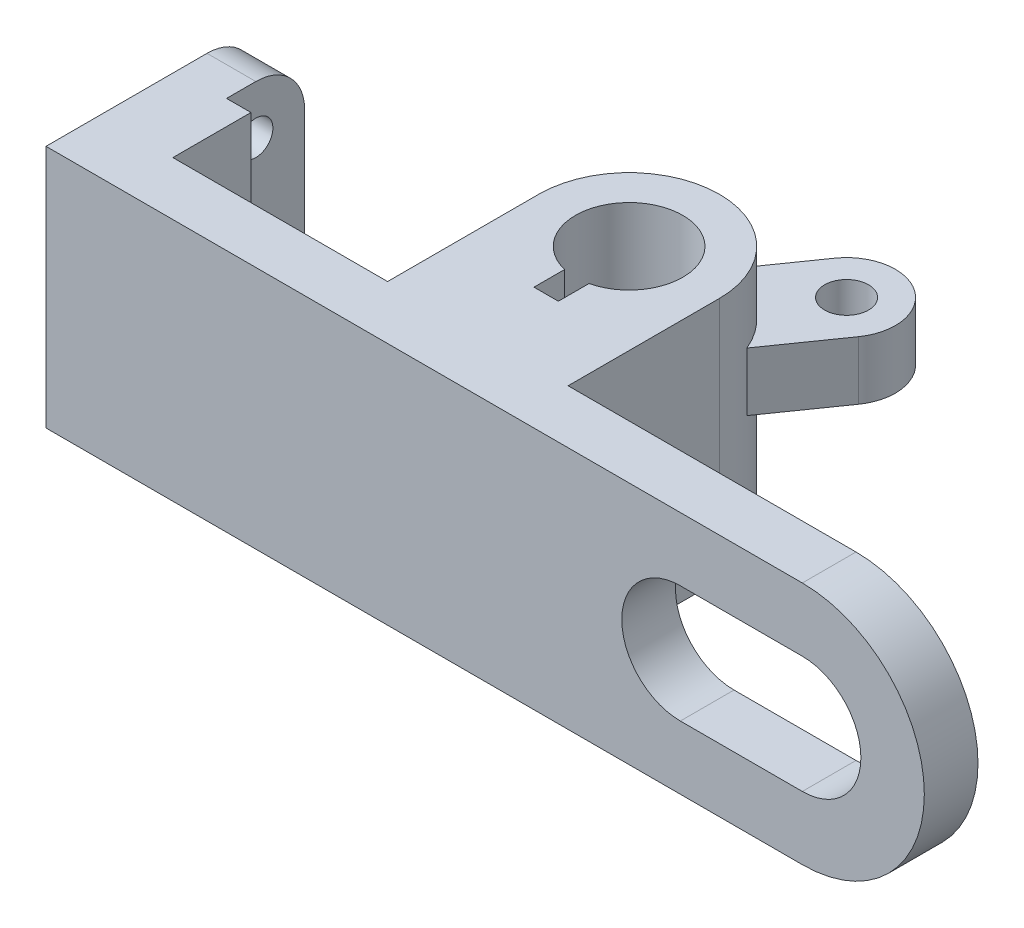
ISO-10303-21;
HEADER;
FILE_DESCRIPTION(('STEP AP214'),'2;1');
FILE_NAME('part.step','',(''),(''),'','','');
FILE_SCHEMA(('AUTOMOTIVE_DESIGN { 1 0 10303 214 1 1 1 1 }'));
ENDSEC;
DATA;
#1=APPLICATION_CONTEXT('core data for automotive mechanical design processes');
#2=APPLICATION_PROTOCOL_DEFINITION('international standard','automotive_design',2000,#1);
#3=PRODUCT_CONTEXT('',#1,'mechanical');
#4=PRODUCT('Part','Part','',(#3));
#5=PRODUCT_RELATED_PRODUCT_CATEGORY('part','',(#4));
#6=PRODUCT_DEFINITION_FORMATION('','',#4);
#7=PRODUCT_DEFINITION_CONTEXT('part definition',#1,'design');
#8=PRODUCT_DEFINITION('design','',#6,#7);
#9=PRODUCT_DEFINITION_SHAPE('','',#8);
#10=(LENGTH_UNIT() NAMED_UNIT(*) SI_UNIT(.MILLI.,.METRE.));
#11=(NAMED_UNIT(*) PLANE_ANGLE_UNIT() SI_UNIT($,.RADIAN.));
#12=(NAMED_UNIT(*) SI_UNIT($,.STERADIAN.) SOLID_ANGLE_UNIT());
#13=UNCERTAINTY_MEASURE_WITH_UNIT(LENGTH_MEASURE(1.E-05),#10,'distance_accuracy_value','');
#14=(GEOMETRIC_REPRESENTATION_CONTEXT(3) GLOBAL_UNCERTAINTY_ASSIGNED_CONTEXT((#13)) GLOBAL_UNIT_ASSIGNED_CONTEXT((#10,
#11,#12)) REPRESENTATION_CONTEXT('',''));
#15=CARTESIAN_POINT('',(0.,0.,0.));
#16=DIRECTION('',(0.,0.,1.));
#17=DIRECTION('',(1.,0.,0.));
#18=AXIS2_PLACEMENT_3D('',#15,#16,#17);
#19=CARTESIAN_POINT('',(0.,25.,-31.));
#20=DIRECTION('',(0.,-1.,0.));
#21=DIRECTION('',(0.,0.,-1.));
#22=AXIS2_PLACEMENT_3D('',#19,#20,#21);
#23=CYLINDRICAL_SURFACE('',#22,18.5);
#24=CARTESIAN_POINT('',(0.,-25.,-31.));
#25=DIRECTION('',(0.,1.,0.));
#26=DIRECTION('',(0.,0.,1.));
#27=AXIS2_PLACEMENT_3D('',#24,#25,#26);
#28=CIRCLE('',#27,18.5);
#29=CARTESIAN_POINT('',(18.5,-25.,-31.));
#30=VERTEX_POINT('',#29);
#31=CARTESIAN_POINT('',(-18.5,-25.,-31.));
#32=VERTEX_POINT('',#31);
#33=EDGE_CURVE('E290',#30,#32,#28,.T.);
#34=ORIENTED_EDGE('',*,*,#33,.T.);
#35=DIRECTION('',(0.,-1.,0.));
#36=VECTOR('',#35,1.);
#37=CARTESIAN_POINT('',(-18.5,25.,-31.));
#38=LINE('',#37,#36);
#39=CARTESIAN_POINT('',(-18.5,25.,-31.));
#40=VERTEX_POINT('',#39);
#41=EDGE_CURVE('E299',#40,#32,#38,.T.);
#42=ORIENTED_EDGE('',*,*,#41,.F.);
#43=CARTESIAN_POINT('',(0.,25.,-31.));
#44=DIRECTION('',(0.,1.,0.));
#45=DIRECTION('',(0.,0.,1.));
#46=AXIS2_PLACEMENT_3D('',#43,#44,#45);
#47=CIRCLE('',#46,18.5);
#48=CARTESIAN_POINT('',(18.5,25.,-31.));
#49=VERTEX_POINT('',#48);
#50=EDGE_CURVE('E270',#49,#40,#47,.T.);
#51=ORIENTED_EDGE('',*,*,#50,.F.);
#52=DIRECTION('',(0.,-1.,0.));
#53=VECTOR('',#52,1.);
#54=CARTESIAN_POINT('',(18.5,25.,-31.));
#55=LINE('',#54,#53);
#56=EDGE_CURVE('E301',#49,#30,#55,.T.);
#57=ORIENTED_EDGE('',*,*,#56,.T.);
#58=EDGE_LOOP('',(#34,#42,#51,#57));
#59=FACE_BOUND('',#58,.T.);
#60=DIRECTION('',(0.,-1.,0.));
#61=VECTOR('',#60,1.);
#62=CARTESIAN_POINT('',(17.1188834432209,12.,-38.0138313108756));
#63=LINE('',#62,#61);
#64=CARTESIAN_POINT('',(17.1188834432209,12.,-38.0138313108756));
#65=VERTEX_POINT('',#64);
#66=CARTESIAN_POINT('',(17.1188834432209,0.,-38.0138313108756));
#67=VERTEX_POINT('',#66);
#68=EDGE_CURVE('E59',#65,#67,#63,.T.);
#69=ORIENTED_EDGE('',*,*,#68,.F.);
#70=CARTESIAN_POINT('',(0.,12.,-31.));
#71=DIRECTION('',(0.,-1.,0.));
#72=DIRECTION('',(0.,0.,1.));
#73=AXIS2_PLACEMENT_3D('',#70,#71,#72);
#74=CIRCLE('',#73,18.5);
#75=CARTESIAN_POINT('',(0.735842557440977,12.,-49.4853600378965));
#76=VERTEX_POINT('',#75);
#77=EDGE_CURVE('E224',#76,#65,#74,.T.);
#78=ORIENTED_EDGE('',*,*,#77,.F.);
#79=DIRECTION('',(0.,-1.,0.));
#80=VECTOR('',#79,1.);
#81=CARTESIAN_POINT('',(0.735842557440977,12.,-49.4853600378965));
#82=LINE('',#81,#80);
#83=CARTESIAN_POINT('',(0.735842557440979,0.,-49.4853600378965));
#84=VERTEX_POINT('',#83);
#85=EDGE_CURVE('E240',#76,#84,#82,.T.);
#86=ORIENTED_EDGE('',*,*,#85,.T.);
#87=CARTESIAN_POINT('',(0.,0.,-31.));
#88=DIRECTION('',(0.,-1.,0.));
#89=DIRECTION('',(0.,0.,1.));
#90=AXIS2_PLACEMENT_3D('',#87,#88,#89);
#91=CIRCLE('',#90,18.5);
#92=EDGE_CURVE('E64',#84,#67,#91,.T.);
#93=ORIENTED_EDGE('',*,*,#92,.T.);
#94=EDGE_LOOP('',(#69,#78,#86,#93));
#95=FACE_BOUND('',#94,.T.);
#96=ADVANCED_FACE('F41',(#59,#95),#23,.T.);
#97=CARTESIAN_POINT('',(77.5,0.,0.));
#98=DIRECTION('',(0.,0.,1.));
#99=DIRECTION('',(1.,0.,0.));
#100=AXIS2_PLACEMENT_3D('',#97,#98,#99);
#101=PLANE('',#100);
#102=CARTESIAN_POINT('',(52.5,0.,0.));
#103=DIRECTION('',(0.,0.,1.));
#104=DIRECTION('',(1.,0.,0.));
#105=AXIS2_PLACEMENT_3D('',#102,#103,#104);
#106=CIRCLE('',#105,12.);
#107=CARTESIAN_POINT('',(52.5,12.,0.));
#108=VERTEX_POINT('',#107);
#109=CARTESIAN_POINT('',(52.5,-12.,0.));
#110=VERTEX_POINT('',#109);
#111=EDGE_CURVE('E347',#108,#110,#106,.T.);
#112=ORIENTED_EDGE('',*,*,#111,.T.);
#113=DIRECTION('',(1.,0.,0.));
#114=VECTOR('',#113,1.);
#115=CARTESIAN_POINT('',(52.5,-12.,0.));
#116=LINE('',#115,#114);
#117=CARTESIAN_POINT('',(77.5,-12.,0.));
#118=VERTEX_POINT('',#117);
#119=EDGE_CURVE('E359',#110,#118,#116,.T.);
#120=ORIENTED_EDGE('',*,*,#119,.T.);
#121=CARTESIAN_POINT('',(77.5,0.,0.));
#122=DIRECTION('',(0.,0.,1.));
#123=DIRECTION('',(1.,0.,0.));
#124=AXIS2_PLACEMENT_3D('',#121,#122,#123);
#125=CIRCLE('',#124,12.);
#126=CARTESIAN_POINT('',(77.5,12.,0.));
#127=VERTEX_POINT('',#126);
#128=EDGE_CURVE('E361',#118,#127,#125,.T.);
#129=ORIENTED_EDGE('',*,*,#128,.T.);
#130=DIRECTION('',(-1.,0.,0.));
#131=VECTOR('',#130,1.);
#132=CARTESIAN_POINT('',(52.5,12.,0.));
#133=LINE('',#132,#131);
#134=EDGE_CURVE('E348',#127,#108,#133,.T.);
#135=ORIENTED_EDGE('',*,*,#134,.T.);
#136=EDGE_LOOP('',(#112,#120,#129,#135));
#137=FACE_BOUND('',#136,.T.);
#138=DIRECTION('',(0.,-1.,0.));
#139=VECTOR('',#138,1.);
#140=CARTESIAN_POINT('',(18.5,25.,0.));
#141=LINE('',#140,#139);
#142=CARTESIAN_POINT('',(18.5,25.,0.));
#143=VERTEX_POINT('',#142);
#144=CARTESIAN_POINT('',(18.5,-25.,0.));
#145=VERTEX_POINT('',#144);
#146=EDGE_CURVE('E291',#143,#145,#141,.T.);
#147=ORIENTED_EDGE('',*,*,#146,.F.);
#148=DIRECTION('',(-1.,0.,0.));
#149=VECTOR('',#148,1.);
#150=CARTESIAN_POINT('',(-77.5,25.,0.));
#151=LINE('',#150,#149);
#152=CARTESIAN_POINT('',(77.5,25.0000000000001,0.));
#153=VERTEX_POINT('',#152);
#154=EDGE_CURVE('E385',#153,#143,#151,.T.);
#155=ORIENTED_EDGE('',*,*,#154,.F.);
#156=CARTESIAN_POINT('',(77.5,0.,0.));
#157=DIRECTION('',(0.,0.,1.));
#158=DIRECTION('',(1.,0.,0.));
#159=AXIS2_PLACEMENT_3D('',#156,#157,#158);
#160=CIRCLE('',#159,25.);
#161=CARTESIAN_POINT('',(77.5,-25.,0.));
#162=VERTEX_POINT('',#161);
#163=EDGE_CURVE('E395',#162,#153,#160,.T.);
#164=ORIENTED_EDGE('',*,*,#163,.F.);
#165=DIRECTION('',(1.,0.,0.));
#166=VECTOR('',#165,1.);
#167=CARTESIAN_POINT('',(-77.5,-25.,0.));
#168=LINE('',#167,#166);
#169=EDGE_CURVE('E380',#145,#162,#168,.T.);
#170=ORIENTED_EDGE('',*,*,#169,.F.);
#171=EDGE_LOOP('',(#147,#155,#164,#170));
#172=FACE_BOUND('',#171,.T.);
#173=ADVANCED_FACE('F480',(#137,#172),#101,.F.);
#174=CARTESIAN_POINT('',(-18.5,25.,0.));
#175=VERTEX_POINT('',#174);
#176=CARTESIAN_POINT('',(-62.5,25.,0.));
#177=VERTEX_POINT('',#176);
#178=EDGE_CURVE('E391',#175,#177,#151,.T.);
#179=ORIENTED_EDGE('',*,*,#178,.F.);
#180=DIRECTION('',(0.,-1.,0.));
#181=VECTOR('',#180,1.);
#182=CARTESIAN_POINT('',(-18.5,25.,0.));
#183=LINE('',#182,#181);
#184=CARTESIAN_POINT('',(-18.5,-25.,0.));
#185=VERTEX_POINT('',#184);
#186=EDGE_CURVE('E294',#175,#185,#183,.T.);
#187=ORIENTED_EDGE('',*,*,#186,.T.);
#188=CARTESIAN_POINT('',(-62.5,-25.,0.));
#189=VERTEX_POINT('',#188);
#190=EDGE_CURVE('E386',#189,#185,#168,.T.);
#191=ORIENTED_EDGE('',*,*,#190,.F.);
#192=DIRECTION('',(0.,-1.,0.));
#193=VECTOR('',#192,1.);
#194=CARTESIAN_POINT('',(-62.5,25.,0.));
#195=LINE('',#194,#193);
#196=EDGE_CURVE('E344',#177,#189,#195,.T.);
#197=ORIENTED_EDGE('',*,*,#196,.F.);
#198=EDGE_LOOP('',(#179,#187,#191,#197));
#199=FACE_BOUND('',#198,.T.);
#200=ADVANCED_FACE('F489',(#199),#101,.F.);
#201=CARTESIAN_POINT('',(77.5,0.,11.));
#202=DIRECTION('',(0.,0.,1.));
#203=DIRECTION('',(1.,0.,0.));
#204=AXIS2_PLACEMENT_3D('',#201,#202,#203);
#205=PLANE('',#204);
#206=DIRECTION('',(0.,-1.,0.));
#207=VECTOR('',#206,1.);
#208=CARTESIAN_POINT('',(-77.5,25.,11.));
#209=LINE('',#208,#207);
#210=CARTESIAN_POINT('',(-77.5,25.,11.));
#211=VERTEX_POINT('',#210);
#212=CARTESIAN_POINT('',(-77.5,-25.,11.));
#213=VERTEX_POINT('',#212);
#214=EDGE_CURVE('E377',#211,#213,#209,.T.);
#215=ORIENTED_EDGE('',*,*,#214,.T.);
#216=DIRECTION('',(1.,0.,0.));
#217=VECTOR('',#216,1.);
#218=CARTESIAN_POINT('',(-77.5,-25.,11.));
#219=LINE('',#218,#217);
#220=CARTESIAN_POINT('',(77.5,-25.,11.));
#221=VERTEX_POINT('',#220);
#222=EDGE_CURVE('E382',#213,#221,#219,.T.);
#223=ORIENTED_EDGE('',*,*,#222,.T.);
#224=CARTESIAN_POINT('',(77.5,0.,11.));
#225=DIRECTION('',(0.,0.,1.));
#226=DIRECTION('',(1.,0.,0.));
#227=AXIS2_PLACEMENT_3D('',#224,#225,#226);
#228=CIRCLE('',#227,25.);
#229=CARTESIAN_POINT('',(77.5,25.0000000000001,11.));
#230=VERTEX_POINT('',#229);
#231=EDGE_CURVE('E381',#221,#230,#228,.T.);
#232=ORIENTED_EDGE('',*,*,#231,.T.);
#233=DIRECTION('',(-1.,0.,0.));
#234=VECTOR('',#233,1.);
#235=CARTESIAN_POINT('',(-77.5,25.,11.));
#236=LINE('',#235,#234);
#237=EDGE_CURVE('E387',#230,#211,#236,.T.);
#238=ORIENTED_EDGE('',*,*,#237,.T.);
#239=EDGE_LOOP('',(#215,#223,#232,#238));
#240=FACE_BOUND('',#239,.T.);
#241=DIRECTION('',(1.,0.,0.));
#242=VECTOR('',#241,1.);
#243=CARTESIAN_POINT('',(52.5,-12.,11.));
#244=LINE('',#243,#242);
#245=CARTESIAN_POINT('',(52.5,-12.,11.));
#246=VERTEX_POINT('',#245);
#247=CARTESIAN_POINT('',(77.5,-12.,11.));
#248=VERTEX_POINT('',#247);
#249=EDGE_CURVE('E346',#246,#248,#244,.T.);
#250=ORIENTED_EDGE('',*,*,#249,.F.);
#251=CARTESIAN_POINT('',(52.5,0.,11.));
#252=DIRECTION('',(0.,0.,1.));
#253=DIRECTION('',(1.,0.,0.));
#254=AXIS2_PLACEMENT_3D('',#251,#252,#253);
#255=CIRCLE('',#254,12.);
#256=CARTESIAN_POINT('',(52.5,12.,11.));
#257=VERTEX_POINT('',#256);
#258=EDGE_CURVE('E350',#257,#246,#255,.T.);
#259=ORIENTED_EDGE('',*,*,#258,.F.);
#260=DIRECTION('',(-1.,0.,0.));
#261=VECTOR('',#260,1.);
#262=CARTESIAN_POINT('',(52.5,12.,11.));
#263=LINE('',#262,#261);
#264=CARTESIAN_POINT('',(77.5,12.,11.));
#265=VERTEX_POINT('',#264);
#266=EDGE_CURVE('E352',#265,#257,#263,.T.);
#267=ORIENTED_EDGE('',*,*,#266,.F.);
#268=CARTESIAN_POINT('',(77.5,0.,11.));
#269=DIRECTION('',(0.,0.,1.));
#270=DIRECTION('',(1.,0.,0.));
#271=AXIS2_PLACEMENT_3D('',#268,#269,#270);
#272=CIRCLE('',#271,12.);
#273=EDGE_CURVE('E351',#248,#265,#272,.T.);
#274=ORIENTED_EDGE('',*,*,#273,.F.);
#275=EDGE_LOOP('',(#250,#259,#267,#274));
#276=FACE_BOUND('',#275,.T.);
#277=ADVANCED_FACE('F437',(#240,#276),#205,.T.);
#278=CARTESIAN_POINT('',(-77.5,25.,11.));
#279=DIRECTION('',(1.,0.,0.));
#280=DIRECTION('',(0.,0.,-1.));
#281=AXIS2_PLACEMENT_3D('',#278,#279,#280);
#282=PLANE('',#281);
#283=CARTESIAN_POINT('',(-77.5,15.,-22.));
#284=DIRECTION('',(1.,0.,0.));
#285=DIRECTION('',(0.,0.,-1.));
#286=AXIS2_PLACEMENT_3D('',#283,#284,#285);
#287=CIRCLE('',#286,3.5);
#288=CARTESIAN_POINT('',(-77.5,15.,-25.5));
#289=VERTEX_POINT('',#288);
#290=EDGE_CURVE('E313',#289,#289,#287,.T.);
#291=ORIENTED_EDGE('',*,*,#290,.T.);
#292=EDGE_LOOP('',(#291));
#293=FACE_BOUND('',#292,.T.);
#294=CARTESIAN_POINT('',(-77.5,-15.,-22.));
#295=DIRECTION('',(1.,0.,0.));
#296=DIRECTION('',(0.,0.,-1.));
#297=AXIS2_PLACEMENT_3D('',#294,#295,#296);
#298=CIRCLE('',#297,3.5);
#299=CARTESIAN_POINT('',(-77.5,-15.,-25.5));
#300=VERTEX_POINT('',#299);
#301=EDGE_CURVE('E311',#300,#300,#298,.T.);
#302=ORIENTED_EDGE('',*,*,#301,.T.);
#303=EDGE_LOOP('',(#302));
#304=FACE_BOUND('',#303,.T.);
#305=DIRECTION('',(0.,0.,-1.));
#306=VECTOR('',#305,1.);
#307=CARTESIAN_POINT('',(-77.5,25.,11.));
#308=LINE('',#307,#306);
#309=CARTESIAN_POINT('',(-77.5,25.,-22.));
#310=VERTEX_POINT('',#309);
#311=EDGE_CURVE('E389',#211,#310,#308,.T.);
#312=ORIENTED_EDGE('',*,*,#311,.T.);
#313=CARTESIAN_POINT('',(-77.5,15.,-22.));
#314=DIRECTION('',(1.,0.,0.));
#315=DIRECTION('',(0.,0.,-1.));
#316=AXIS2_PLACEMENT_3D('',#313,#314,#315);
#317=CIRCLE('',#316,10.);
#318=CARTESIAN_POINT('',(-77.5,15.,-32.));
#319=VERTEX_POINT('',#318);
#320=EDGE_CURVE('E414',#310,#319,#317,.F.);
#321=ORIENTED_EDGE('',*,*,#320,.T.);
#322=DIRECTION('',(0.,-1.,0.));
#323=VECTOR('',#322,1.);
#324=CARTESIAN_POINT('',(-77.5,25.,-32.));
#325=LINE('',#324,#323);
#326=CARTESIAN_POINT('',(-77.5,-15.,-32.));
#327=VERTEX_POINT('',#326);
#328=EDGE_CURVE('E327',#319,#327,#325,.T.);
#329=ORIENTED_EDGE('',*,*,#328,.T.);
#330=CARTESIAN_POINT('',(-77.5,-15.,-22.));
#331=DIRECTION('',(1.,0.,0.));
#332=DIRECTION('',(0.,0.,-1.));
#333=AXIS2_PLACEMENT_3D('',#330,#331,#332);
#334=CIRCLE('',#333,10.);
#335=CARTESIAN_POINT('',(-77.5,-25.,-22.));
#336=VERTEX_POINT('',#335);
#337=EDGE_CURVE('E412',#327,#336,#334,.F.);
#338=ORIENTED_EDGE('',*,*,#337,.T.);
#339=DIRECTION('',(0.,0.,-1.));
#340=VECTOR('',#339,1.);
#341=CARTESIAN_POINT('',(-77.5,-25.,11.));
#342=LINE('',#341,#340);
#343=EDGE_CURVE('E403',#213,#336,#342,.T.);
#344=ORIENTED_EDGE('',*,*,#343,.F.);
#345=ORIENTED_EDGE('',*,*,#214,.F.);
#346=EDGE_LOOP('',(#312,#321,#329,#338,#344,#345));
#347=FACE_BOUND('',#346,.T.);
#348=ADVANCED_FACE('F434',(#293,#304,#347),#282,.F.);
#349=CARTESIAN_POINT('',(-77.5,-25.,11.));
#350=DIRECTION('',(0.,1.,0.));
#351=DIRECTION('',(-1.,0.,0.));
#352=AXIS2_PLACEMENT_3D('',#349,#350,#351);
#353=PLANE('',#352);
#354=ORIENTED_EDGE('',*,*,#343,.T.);
#355=DIRECTION('',(-1.,0.,0.));
#356=VECTOR('',#355,1.);
#357=CARTESIAN_POINT('',(-77.5,-25.,-22.));
#358=LINE('',#357,#356);
#359=CARTESIAN_POINT('',(-67.5,-25.,-22.));
#360=VERTEX_POINT('',#359);
#361=EDGE_CURVE('E11',#336,#360,#358,.F.);
#362=ORIENTED_EDGE('',*,*,#361,.T.);
#363=DIRECTION('',(0.,0.,-1.));
#364=VECTOR('',#363,1.);
#365=CARTESIAN_POINT('',(-67.5,-25.,-32.));
#366=LINE('',#365,#364);
#367=CARTESIAN_POINT('',(-67.5,-25.,-16.));
#368=VERTEX_POINT('',#367);
#369=EDGE_CURVE('E322',#368,#360,#366,.T.);
#370=ORIENTED_EDGE('',*,*,#369,.F.);
#371=DIRECTION('',(-1.,0.,0.));
#372=VECTOR('',#371,1.);
#373=CARTESIAN_POINT('',(-67.5,-25.,-16.));
#374=LINE('',#373,#372);
#375=CARTESIAN_POINT('',(-62.5,-25.,-16.));
#376=VERTEX_POINT('',#375);
#377=EDGE_CURVE('E329',#376,#368,#374,.T.);
#378=ORIENTED_EDGE('',*,*,#377,.F.);
#379=DIRECTION('',(0.,0.,-1.));
#380=VECTOR('',#379,1.);
#381=CARTESIAN_POINT('',(-62.5,-25.,-16.));
#382=LINE('',#381,#380);
#383=EDGE_CURVE('E320',#189,#376,#382,.T.);
#384=ORIENTED_EDGE('',*,*,#383,.F.);
#385=ORIENTED_EDGE('',*,*,#190,.T.);
#386=DIRECTION('',(0.,0.,-1.));
#387=VECTOR('',#386,1.);
#388=CARTESIAN_POINT('',(-18.5,-25.,0.));
#389=LINE('',#388,#387);
#390=EDGE_CURVE('E260',#185,#32,#389,.T.);
#391=ORIENTED_EDGE('',*,*,#390,.T.);
#392=ORIENTED_EDGE('',*,*,#33,.F.);
#393=DIRECTION('',(0.,0.,-1.));
#394=VECTOR('',#393,1.);
#395=CARTESIAN_POINT('',(18.5,-25.,0.));
#396=LINE('',#395,#394);
#397=EDGE_CURVE('E283',#145,#30,#396,.T.);
#398=ORIENTED_EDGE('',*,*,#397,.F.);
#399=ORIENTED_EDGE('',*,*,#169,.T.);
#400=DIRECTION('',(0.,0.,-1.));
#401=VECTOR('',#400,1.);
#402=CARTESIAN_POINT('',(77.5,-25.,11.));
#403=LINE('',#402,#401);
#404=EDGE_CURVE('E405',#221,#162,#403,.T.);
#405=ORIENTED_EDGE('',*,*,#404,.F.);
#406=ORIENTED_EDGE('',*,*,#222,.F.);
#407=EDGE_LOOP('',(#354,#362,#370,#378,#384,#385,#391,#392,#398,#399,#405,#406));
#408=FACE_BOUND('',#407,.T.);
#409=CARTESIAN_POINT('',(0.,-25.,-31.));
#410=DIRECTION('',(0.,1.,0.));
#411=DIRECTION('',(0.,0.,1.));
#412=AXIS2_PLACEMENT_3D('',#409,#410,#411);
#413=CIRCLE('',#412,11.);
#414=CARTESIAN_POINT('',(2.49999999999999,-25.,-20.2878573571858));
#415=VERTEX_POINT('',#414);
#416=CARTESIAN_POINT('',(-2.50000000000001,-25.,-20.2878573571858));
#417=VERTEX_POINT('',#416);
#418=EDGE_CURVE('E255',#415,#417,#413,.T.);
#419=ORIENTED_EDGE('',*,*,#418,.T.);
#420=DIRECTION('',(0.,0.,-1.));
#421=VECTOR('',#420,1.);
#422=CARTESIAN_POINT('',(-2.49999999999984,-25.,0.));
#423=LINE('',#422,#421);
#424=CARTESIAN_POINT('',(-2.49999999999996,-25.,-14.));
#425=VERTEX_POINT('',#424);
#426=EDGE_CURVE('E285',#425,#417,#423,.T.);
#427=ORIENTED_EDGE('',*,*,#426,.F.);
#428=DIRECTION('',(1.,0.,0.));
#429=VECTOR('',#428,1.);
#430=CARTESIAN_POINT('',(0.,-25.,-14.));
#431=LINE('',#430,#429);
#432=CARTESIAN_POINT('',(2.50000000000004,-25.,-14.));
#433=VERTEX_POINT('',#432);
#434=EDGE_CURVE('E276',#425,#433,#431,.T.);
#435=ORIENTED_EDGE('',*,*,#434,.T.);
#436=DIRECTION('',(0.,0.,-1.));
#437=VECTOR('',#436,1.);
#438=CARTESIAN_POINT('',(2.50000000000016,-25.,0.));
#439=LINE('',#438,#437);
#440=EDGE_CURVE('E277',#433,#415,#439,.T.);
#441=ORIENTED_EDGE('',*,*,#440,.T.);
#442=EDGE_LOOP('',(#419,#427,#435,#441));
#443=FACE_BOUND('',#442,.T.);
#444=ADVANCED_FACE('F438',(#408,#443),#353,.F.);
#445=CARTESIAN_POINT('',(77.5,0.,11.));
#446=DIRECTION('',(0.,0.,-1.));
#447=DIRECTION('',(-1.,0.,0.));
#448=AXIS2_PLACEMENT_3D('',#445,#446,#447);
#449=CYLINDRICAL_SURFACE('',#448,25.);
#450=ORIENTED_EDGE('',*,*,#163,.T.);
#451=DIRECTION('',(0.,0.,-1.));
#452=VECTOR('',#451,1.);
#453=CARTESIAN_POINT('',(77.5,25.0000000000001,11.));
#454=LINE('',#453,#452);
#455=EDGE_CURVE('E398',#230,#153,#454,.T.);
#456=ORIENTED_EDGE('',*,*,#455,.F.);
#457=ORIENTED_EDGE('',*,*,#231,.F.);
#458=ORIENTED_EDGE('',*,*,#404,.T.);
#459=EDGE_LOOP('',(#450,#456,#457,#458));
#460=FACE_BOUND('',#459,.T.);
#461=ADVANCED_FACE('F475',(#460),#449,.T.);
#462=CARTESIAN_POINT('',(-77.5,25.,11.));
#463=DIRECTION('',(0.,-1.,0.));
#464=DIRECTION('',(1.,0.,0.));
#465=AXIS2_PLACEMENT_3D('',#462,#463,#464);
#466=PLANE('',#465);
#467=DIRECTION('',(0.,0.,-1.));
#468=VECTOR('',#467,1.);
#469=CARTESIAN_POINT('',(-67.5,25.,-32.));
#470=LINE('',#469,#468);
#471=CARTESIAN_POINT('',(-67.5,25.,-16.));
#472=VERTEX_POINT('',#471);
#473=CARTESIAN_POINT('',(-67.5,25.,-22.));
#474=VERTEX_POINT('',#473);
#475=EDGE_CURVE('E324',#472,#474,#470,.T.);
#476=ORIENTED_EDGE('',*,*,#475,.T.);
#477=DIRECTION('',(-1.,0.,0.));
#478=VECTOR('',#477,1.);
#479=CARTESIAN_POINT('',(-77.5,25.,-22.));
#480=LINE('',#479,#478);
#481=EDGE_CURVE('E409',#474,#310,#480,.T.);
#482=ORIENTED_EDGE('',*,*,#481,.T.);
#483=ORIENTED_EDGE('',*,*,#311,.F.);
#484=ORIENTED_EDGE('',*,*,#237,.F.);
#485=ORIENTED_EDGE('',*,*,#455,.T.);
#486=ORIENTED_EDGE('',*,*,#154,.T.);
#487=DIRECTION('',(0.,0.,-1.));
#488=VECTOR('',#487,1.);
#489=CARTESIAN_POINT('',(18.5,25.,0.));
#490=LINE('',#489,#488);
#491=EDGE_CURVE('E263',#143,#49,#490,.T.);
#492=ORIENTED_EDGE('',*,*,#491,.T.);
#493=ORIENTED_EDGE('',*,*,#50,.T.);
#494=DIRECTION('',(0.,0.,-1.));
#495=VECTOR('',#494,1.);
#496=CARTESIAN_POINT('',(-18.5,25.,0.));
#497=LINE('',#496,#495);
#498=EDGE_CURVE('E267',#175,#40,#497,.T.);
#499=ORIENTED_EDGE('',*,*,#498,.F.);
#500=ORIENTED_EDGE('',*,*,#178,.T.);
#501=DIRECTION('',(0.,0.,-1.));
#502=VECTOR('',#501,1.);
#503=CARTESIAN_POINT('',(-62.5,25.,-16.));
#504=LINE('',#503,#502);
#505=CARTESIAN_POINT('',(-62.5,25.,-16.));
#506=VERTEX_POINT('',#505);
#507=EDGE_CURVE('E319',#177,#506,#504,.T.);
#508=ORIENTED_EDGE('',*,*,#507,.T.);
#509=DIRECTION('',(-1.,0.,0.));
#510=VECTOR('',#509,1.);
#511=CARTESIAN_POINT('',(-67.5,25.,-16.));
#512=LINE('',#511,#510);
#513=EDGE_CURVE('E318',#506,#472,#512,.T.);
#514=ORIENTED_EDGE('',*,*,#513,.T.);
#515=EDGE_LOOP('',(#476,#482,#483,#484,#485,#486,#492,#493,#499,#500,#508,#514));
#516=FACE_BOUND('',#515,.T.);
#517=CARTESIAN_POINT('',(0.,25.,-31.));
#518=DIRECTION('',(0.,1.,0.));
#519=DIRECTION('',(0.,0.,1.));
#520=AXIS2_PLACEMENT_3D('',#517,#518,#519);
#521=CIRCLE('',#520,11.);
#522=CARTESIAN_POINT('',(2.49999999999999,25.,-20.2878573571858));
#523=VERTEX_POINT('',#522);
#524=CARTESIAN_POINT('',(-2.50000000000001,25.,-20.2878573571858));
#525=VERTEX_POINT('',#524);
#526=EDGE_CURVE('E254',#523,#525,#521,.T.);
#527=ORIENTED_EDGE('',*,*,#526,.F.);
#528=DIRECTION('',(0.,0.,-1.));
#529=VECTOR('',#528,1.);
#530=CARTESIAN_POINT('',(2.50000000000016,25.,0.));
#531=LINE('',#530,#529);
#532=CARTESIAN_POINT('',(2.50000000000004,25.,-14.));
#533=VERTEX_POINT('',#532);
#534=EDGE_CURVE('E257',#533,#523,#531,.T.);
#535=ORIENTED_EDGE('',*,*,#534,.F.);
#536=DIRECTION('',(1.,0.,0.));
#537=VECTOR('',#536,1.);
#538=CARTESIAN_POINT('',(0.,25.,-14.));
#539=LINE('',#538,#537);
#540=CARTESIAN_POINT('',(-2.49999999999996,25.,-14.));
#541=VERTEX_POINT('',#540);
#542=EDGE_CURVE('E258',#541,#533,#539,.T.);
#543=ORIENTED_EDGE('',*,*,#542,.F.);
#544=DIRECTION('',(0.,0.,-1.));
#545=VECTOR('',#544,1.);
#546=CARTESIAN_POINT('',(-2.49999999999984,25.,0.));
#547=LINE('',#546,#545);
#548=EDGE_CURVE('E264',#541,#525,#547,.T.);
#549=ORIENTED_EDGE('',*,*,#548,.T.);
#550=EDGE_LOOP('',(#527,#535,#543,#549));
#551=FACE_BOUND('',#550,.T.);
#552=ADVANCED_FACE('F449',(#516,#551),#466,.F.);
#553=CARTESIAN_POINT('',(52.5,0.,11.));
#554=DIRECTION('',(0.,0.,-1.));
#555=DIRECTION('',(-1.,0.,0.));
#556=AXIS2_PLACEMENT_3D('',#553,#554,#555);
#557=CYLINDRICAL_SURFACE('',#556,12.);
#558=ORIENTED_EDGE('',*,*,#111,.F.);
#559=DIRECTION('',(0.,0.,-1.));
#560=VECTOR('',#559,1.);
#561=CARTESIAN_POINT('',(52.5,12.,11.));
#562=LINE('',#561,#560);
#563=EDGE_CURVE('E357',#257,#108,#562,.T.);
#564=ORIENTED_EDGE('',*,*,#563,.F.);
#565=ORIENTED_EDGE('',*,*,#258,.T.);
#566=DIRECTION('',(0.,0.,-1.));
#567=VECTOR('',#566,1.);
#568=CARTESIAN_POINT('',(52.5,-12.,11.));
#569=LINE('',#568,#567);
#570=EDGE_CURVE('E372',#246,#110,#569,.T.);
#571=ORIENTED_EDGE('',*,*,#570,.T.);
#572=EDGE_LOOP('',(#558,#564,#565,#571));
#573=FACE_BOUND('',#572,.T.);
#574=ADVANCED_FACE('F560',(#573),#557,.F.);
#575=CARTESIAN_POINT('',(52.5,-12.,11.));
#576=DIRECTION('',(0.,1.,0.));
#577=DIRECTION('',(-1.,0.,0.));
#578=AXIS2_PLACEMENT_3D('',#575,#576,#577);
#579=PLANE('',#578);
#580=ORIENTED_EDGE('',*,*,#119,.F.);
#581=ORIENTED_EDGE('',*,*,#570,.F.);
#582=ORIENTED_EDGE('',*,*,#249,.T.);
#583=DIRECTION('',(0.,0.,-1.));
#584=VECTOR('',#583,1.);
#585=CARTESIAN_POINT('',(77.5,-12.,11.));
#586=LINE('',#585,#584);
#587=EDGE_CURVE('E375',#248,#118,#586,.T.);
#588=ORIENTED_EDGE('',*,*,#587,.T.);
#589=EDGE_LOOP('',(#580,#581,#582,#588));
#590=FACE_BOUND('',#589,.T.);
#591=ADVANCED_FACE('F562',(#590),#579,.T.);
#592=CARTESIAN_POINT('',(77.5,0.,11.));
#593=DIRECTION('',(0.,0.,-1.));
#594=DIRECTION('',(-1.,0.,0.));
#595=AXIS2_PLACEMENT_3D('',#592,#593,#594);
#596=CYLINDRICAL_SURFACE('',#595,12.);
#597=ORIENTED_EDGE('',*,*,#128,.F.);
#598=ORIENTED_EDGE('',*,*,#587,.F.);
#599=ORIENTED_EDGE('',*,*,#273,.T.);
#600=DIRECTION('',(0.,0.,-1.));
#601=VECTOR('',#600,1.);
#602=CARTESIAN_POINT('',(77.5,12.,11.));
#603=LINE('',#602,#601);
#604=EDGE_CURVE('E369',#265,#127,#603,.T.);
#605=ORIENTED_EDGE('',*,*,#604,.T.);
#606=EDGE_LOOP('',(#597,#598,#599,#605));
#607=FACE_BOUND('',#606,.T.);
#608=ADVANCED_FACE('F568',(#607),#596,.F.);
#609=CARTESIAN_POINT('',(52.5,12.,11.));
#610=DIRECTION('',(0.,-1.,0.));
#611=DIRECTION('',(1.,0.,0.));
#612=AXIS2_PLACEMENT_3D('',#609,#610,#611);
#613=PLANE('',#612);
#614=ORIENTED_EDGE('',*,*,#134,.F.);
#615=ORIENTED_EDGE('',*,*,#604,.F.);
#616=ORIENTED_EDGE('',*,*,#266,.T.);
#617=ORIENTED_EDGE('',*,*,#563,.T.);
#618=EDGE_LOOP('',(#614,#615,#616,#617));
#619=FACE_BOUND('',#618,.T.);
#620=ADVANCED_FACE('F509',(#619),#613,.T.);
#621=CARTESIAN_POINT('',(-62.5,25.,-16.));
#622=DIRECTION('',(-1.,0.,0.));
#623=DIRECTION('',(0.,0.,1.));
#624=AXIS2_PLACEMENT_3D('',#621,#622,#623);
#625=PLANE('',#624);
#626=ORIENTED_EDGE('',*,*,#383,.T.);
#627=DIRECTION('',(0.,-1.,0.));
#628=VECTOR('',#627,1.);
#629=CARTESIAN_POINT('',(-62.5,25.,-16.));
#630=LINE('',#629,#628);
#631=EDGE_CURVE('E338',#506,#376,#630,.T.);
#632=ORIENTED_EDGE('',*,*,#631,.F.);
#633=ORIENTED_EDGE('',*,*,#507,.F.);
#634=ORIENTED_EDGE('',*,*,#196,.T.);
#635=EDGE_LOOP('',(#626,#632,#633,#634));
#636=FACE_BOUND('',#635,.T.);
#637=ADVANCED_FACE('F492',(#636),#625,.F.);
#638=CARTESIAN_POINT('',(-67.5,25.,-16.));
#639=DIRECTION('',(0.,0.,1.));
#640=DIRECTION('',(1.,0.,0.));
#641=AXIS2_PLACEMENT_3D('',#638,#639,#640);
#642=PLANE('',#641);
#643=ORIENTED_EDGE('',*,*,#377,.T.);
#644=DIRECTION('',(0.,-1.,0.));
#645=VECTOR('',#644,1.);
#646=CARTESIAN_POINT('',(-67.5,25.,-16.));
#647=LINE('',#646,#645);
#648=EDGE_CURVE('E340',#472,#368,#647,.T.);
#649=ORIENTED_EDGE('',*,*,#648,.F.);
#650=ORIENTED_EDGE('',*,*,#513,.F.);
#651=ORIENTED_EDGE('',*,*,#631,.T.);
#652=EDGE_LOOP('',(#643,#649,#650,#651));
#653=FACE_BOUND('',#652,.T.);
#654=ADVANCED_FACE('F497',(#653),#642,.F.);
#655=CARTESIAN_POINT('',(-67.5,25.,-32.));
#656=DIRECTION('',(-1.,0.,0.));
#657=DIRECTION('',(0.,0.,1.));
#658=AXIS2_PLACEMENT_3D('',#655,#656,#657);
#659=PLANE('',#658);
#660=CARTESIAN_POINT('',(-67.5,15.,-22.));
#661=DIRECTION('',(-1.,0.,0.));
#662=DIRECTION('',(0.,0.,1.));
#663=AXIS2_PLACEMENT_3D('',#660,#661,#662);
#664=CIRCLE('',#663,3.5);
#665=CARTESIAN_POINT('',(-67.5,15.,-18.5));
#666=VERTEX_POINT('',#665);
#667=EDGE_CURVE('E44',#666,#666,#664,.T.);
#668=ORIENTED_EDGE('',*,*,#667,.T.);
#669=EDGE_LOOP('',(#668));
#670=FACE_BOUND('',#669,.T.);
#671=CARTESIAN_POINT('',(-67.5,-15.,-22.));
#672=DIRECTION('',(-1.,0.,0.));
#673=DIRECTION('',(0.,0.,1.));
#674=AXIS2_PLACEMENT_3D('',#671,#672,#673);
#675=CIRCLE('',#674,3.5);
#676=CARTESIAN_POINT('',(-67.5,-15.,-18.5));
#677=VERTEX_POINT('',#676);
#678=EDGE_CURVE('E302',#677,#677,#675,.T.);
#679=ORIENTED_EDGE('',*,*,#678,.T.);
#680=EDGE_LOOP('',(#679));
#681=FACE_BOUND('',#680,.T.);
#682=DIRECTION('',(0.,-1.,0.));
#683=VECTOR('',#682,1.);
#684=CARTESIAN_POINT('',(-67.5,25.,-32.));
#685=LINE('',#684,#683);
#686=CARTESIAN_POINT('',(-67.5,15.,-32.));
#687=VERTEX_POINT('',#686);
#688=CARTESIAN_POINT('',(-67.5,-15.,-32.));
#689=VERTEX_POINT('',#688);
#690=EDGE_CURVE('E333',#687,#689,#685,.T.);
#691=ORIENTED_EDGE('',*,*,#690,.F.);
#692=CARTESIAN_POINT('',(-67.5,15.,-22.));
#693=DIRECTION('',(-1.,0.,0.));
#694=DIRECTION('',(0.,0.,1.));
#695=AXIS2_PLACEMENT_3D('',#692,#693,#694);
#696=CIRCLE('',#695,10.);
#697=EDGE_CURVE('E49',#687,#474,#696,.F.);
#698=ORIENTED_EDGE('',*,*,#697,.T.);
#699=ORIENTED_EDGE('',*,*,#475,.F.);
#700=ORIENTED_EDGE('',*,*,#648,.T.);
#701=ORIENTED_EDGE('',*,*,#369,.T.);
#702=CARTESIAN_POINT('',(-67.5,-15.,-22.));
#703=DIRECTION('',(-1.,0.,0.));
#704=DIRECTION('',(0.,0.,1.));
#705=AXIS2_PLACEMENT_3D('',#702,#703,#704);
#706=CIRCLE('',#705,10.);
#707=EDGE_CURVE('E417',#360,#689,#706,.F.);
#708=ORIENTED_EDGE('',*,*,#707,.T.);
#709=EDGE_LOOP('',(#691,#698,#699,#700,#701,#708));
#710=FACE_BOUND('',#709,.T.);
#711=ADVANCED_FACE('F424',(#670,#681,#710),#659,.F.);
#712=CARTESIAN_POINT('',(-77.5,25.,-32.));
#713=DIRECTION('',(0.,0.,1.));
#714=DIRECTION('',(1.,0.,0.));
#715=AXIS2_PLACEMENT_3D('',#712,#713,#714);
#716=PLANE('',#715);
#717=ORIENTED_EDGE('',*,*,#328,.F.);
#718=DIRECTION('',(-1.,0.,0.));
#719=VECTOR('',#718,1.);
#720=CARTESIAN_POINT('',(-77.5,15.,-32.));
#721=LINE('',#720,#719);
#722=EDGE_CURVE('E420',#319,#687,#721,.F.);
#723=ORIENTED_EDGE('',*,*,#722,.T.);
#724=ORIENTED_EDGE('',*,*,#690,.T.);
#725=DIRECTION('',(-1.,0.,0.));
#726=VECTOR('',#725,1.);
#727=CARTESIAN_POINT('',(-77.5,-15.,-32.));
#728=LINE('',#727,#726);
#729=EDGE_CURVE('E413',#689,#327,#728,.T.);
#730=ORIENTED_EDGE('',*,*,#729,.T.);
#731=EDGE_LOOP('',(#717,#723,#724,#730));
#732=FACE_BOUND('',#731,.T.);
#733=ADVANCED_FACE('F459',(#732),#716,.F.);
#734=CARTESIAN_POINT('',(-77.5,15.,-22.));
#735=DIRECTION('',(-1.,0.,0.));
#736=DIRECTION('',(0.,-1.,0.));
#737=AXIS2_PLACEMENT_3D('',#734,#735,#736);
#738=CYLINDRICAL_SURFACE('',#737,10.);
#739=ORIENTED_EDGE('',*,*,#697,.F.);
#740=ORIENTED_EDGE('',*,*,#722,.F.);
#741=ORIENTED_EDGE('',*,*,#320,.F.);
#742=ORIENTED_EDGE('',*,*,#481,.F.);
#743=EDGE_LOOP('',(#739,#740,#741,#742));
#744=FACE_BOUND('',#743,.T.);
#745=ADVANCED_FACE('F451',(#744),#738,.T.);
#746=CARTESIAN_POINT('',(-77.5,-15.,-22.));
#747=DIRECTION('',(-1.,0.,0.));
#748=DIRECTION('',(0.,-1.,0.));
#749=AXIS2_PLACEMENT_3D('',#746,#747,#748);
#750=CYLINDRICAL_SURFACE('',#749,10.);
#751=ORIENTED_EDGE('',*,*,#707,.F.);
#752=ORIENTED_EDGE('',*,*,#361,.F.);
#753=ORIENTED_EDGE('',*,*,#337,.F.);
#754=ORIENTED_EDGE('',*,*,#729,.F.);
#755=EDGE_LOOP('',(#751,#752,#753,#754));
#756=FACE_BOUND('',#755,.T.);
#757=ADVANCED_FACE('F43',(#756),#750,.T.);
#758=CARTESIAN_POINT('',(-52.5,-15.,-22.));
#759=DIRECTION('',(-1.,0.,0.));
#760=DIRECTION('',(0.,0.,1.));
#761=AXIS2_PLACEMENT_3D('',#758,#759,#760);
#762=CYLINDRICAL_SURFACE('',#761,3.5);
#763=ORIENTED_EDGE('',*,*,#678,.F.);
#764=EDGE_LOOP('',(#763));
#765=FACE_BOUND('',#764,.T.);
#766=ORIENTED_EDGE('',*,*,#301,.F.);
#767=EDGE_LOOP('',(#766));
#768=FACE_BOUND('',#767,.T.);
#769=ADVANCED_FACE('F426',(#765,#768),#762,.F.);
#770=CARTESIAN_POINT('',(-52.5,15.,-22.));
#771=DIRECTION('',(-1.,0.,0.));
#772=DIRECTION('',(0.,0.,1.));
#773=AXIS2_PLACEMENT_3D('',#770,#771,#772);
#774=CYLINDRICAL_SURFACE('',#773,3.5);
#775=ORIENTED_EDGE('',*,*,#667,.F.);
#776=EDGE_LOOP('',(#775));
#777=FACE_BOUND('',#776,.T.);
#778=ORIENTED_EDGE('',*,*,#290,.F.);
#779=EDGE_LOOP('',(#778));
#780=FACE_BOUND('',#779,.T.);
#781=ADVANCED_FACE('F431',(#777,#780),#774,.F.);
#782=CARTESIAN_POINT('',(18.5,25.,0.));
#783=DIRECTION('',(-1.,0.,0.));
#784=DIRECTION('',(0.,0.,1.));
#785=AXIS2_PLACEMENT_3D('',#782,#783,#784);
#786=PLANE('',#785);
#787=ORIENTED_EDGE('',*,*,#397,.T.);
#788=ORIENTED_EDGE('',*,*,#56,.F.);
#789=ORIENTED_EDGE('',*,*,#491,.F.);
#790=ORIENTED_EDGE('',*,*,#146,.T.);
#791=EDGE_LOOP('',(#787,#788,#789,#790));
#792=FACE_BOUND('',#791,.T.);
#793=ADVANCED_FACE('F484',(#792),#786,.F.);
#794=CARTESIAN_POINT('',(-18.5,25.,0.));
#795=DIRECTION('',(-1.,0.,0.));
#796=DIRECTION('',(0.,0.,1.));
#797=AXIS2_PLACEMENT_3D('',#794,#795,#796);
#798=PLANE('',#797);
#799=ORIENTED_EDGE('',*,*,#390,.F.);
#800=ORIENTED_EDGE('',*,*,#186,.F.);
#801=ORIENTED_EDGE('',*,*,#498,.T.);
#802=ORIENTED_EDGE('',*,*,#41,.T.);
#803=EDGE_LOOP('',(#799,#800,#801,#802));
#804=FACE_BOUND('',#803,.T.);
#805=ADVANCED_FACE('F524',(#804),#798,.T.);
#806=CARTESIAN_POINT('',(0.,25.,-31.));
#807=DIRECTION('',(0.,-1.,0.));
#808=DIRECTION('',(0.,0.,-1.));
#809=AXIS2_PLACEMENT_3D('',#806,#807,#808);
#810=CYLINDRICAL_SURFACE('',#809,11.);
#811=ORIENTED_EDGE('',*,*,#418,.F.);
#812=DIRECTION('',(0.,-1.,0.));
#813=VECTOR('',#812,1.);
#814=CARTESIAN_POINT('',(2.49999999999999,25.,-20.2878573571858));
#815=LINE('',#814,#813);
#816=EDGE_CURVE('E298',#523,#415,#815,.T.);
#817=ORIENTED_EDGE('',*,*,#816,.F.);
#818=ORIENTED_EDGE('',*,*,#526,.T.);
#819=DIRECTION('',(0.,-1.,0.));
#820=VECTOR('',#819,1.);
#821=CARTESIAN_POINT('',(-2.50000000000001,25.,-20.2878573571858));
#822=LINE('',#821,#820);
#823=EDGE_CURVE('E271',#525,#417,#822,.T.);
#824=ORIENTED_EDGE('',*,*,#823,.T.);
#825=EDGE_LOOP('',(#811,#817,#818,#824));
#826=FACE_BOUND('',#825,.T.);
#827=ADVANCED_FACE('F540',(#826),#810,.F.);
#828=CARTESIAN_POINT('',(2.50000000000016,25.,0.));
#829=DIRECTION('',(-1.,0.,0.));
#830=DIRECTION('',(0.,0.,1.));
#831=AXIS2_PLACEMENT_3D('',#828,#829,#830);
#832=PLANE('',#831);
#833=ORIENTED_EDGE('',*,*,#440,.F.);
#834=DIRECTION('',(0.,-1.,0.));
#835=VECTOR('',#834,1.);
#836=CARTESIAN_POINT('',(2.50000000000004,25.,-14.));
#837=LINE('',#836,#835);
#838=EDGE_CURVE('E308',#533,#433,#837,.T.);
#839=ORIENTED_EDGE('',*,*,#838,.F.);
#840=ORIENTED_EDGE('',*,*,#534,.T.);
#841=ORIENTED_EDGE('',*,*,#816,.T.);
#842=EDGE_LOOP('',(#833,#839,#840,#841));
#843=FACE_BOUND('',#842,.T.);
#844=ADVANCED_FACE('F531',(#843),#832,.T.);
#845=CARTESIAN_POINT('',(0.,25.,-14.));
#846=DIRECTION('',(0.,0.,-1.));
#847=DIRECTION('',(-1.,0.,0.));
#848=AXIS2_PLACEMENT_3D('',#845,#846,#847);
#849=PLANE('',#848);
#850=ORIENTED_EDGE('',*,*,#434,.F.);
#851=DIRECTION('',(0.,-1.,0.));
#852=VECTOR('',#851,1.);
#853=CARTESIAN_POINT('',(-2.49999999999996,25.,-14.));
#854=LINE('',#853,#852);
#855=EDGE_CURVE('E306',#541,#425,#854,.T.);
#856=ORIENTED_EDGE('',*,*,#855,.F.);
#857=ORIENTED_EDGE('',*,*,#542,.T.);
#858=ORIENTED_EDGE('',*,*,#838,.T.);
#859=EDGE_LOOP('',(#850,#856,#857,#858));
#860=FACE_BOUND('',#859,.T.);
#861=ADVANCED_FACE('F528',(#860),#849,.T.);
#862=CARTESIAN_POINT('',(-2.49999999999984,25.,0.));
#863=DIRECTION('',(-1.,0.,0.));
#864=DIRECTION('',(0.,0.,1.));
#865=AXIS2_PLACEMENT_3D('',#862,#863,#864);
#866=PLANE('',#865);
#867=ORIENTED_EDGE('',*,*,#426,.T.);
#868=ORIENTED_EDGE('',*,*,#823,.F.);
#869=ORIENTED_EDGE('',*,*,#548,.F.);
#870=ORIENTED_EDGE('',*,*,#855,.T.);
#871=EDGE_LOOP('',(#867,#868,#869,#870));
#872=FACE_BOUND('',#871,.T.);
#873=ADVANCED_FACE('F526',(#872),#866,.F.);
#874=CARTESIAN_POINT('',(0.,12.,-31.));
#875=DIRECTION('',(0.,1.,0.));
#876=DIRECTION('',(0.,0.,1.));
#877=AXIS2_PLACEMENT_3D('',#874,#875,#876);
#878=PLANE('',#877);
#879=ORIENTED_EDGE('',*,*,#77,.T.);
#880=DIRECTION('',(0.573576436351044,0.,-0.819152044288993));
#881=VECTOR('',#880,1.);
#882=CARTESIAN_POINT('',(17.1188834432209,12.,-38.0138313108756));
#883=LINE('',#882,#881);
#884=CARTESIAN_POINT('',(26.5459664061233,12.,-51.4771010537374));
#885=VERTEX_POINT('',#884);
#886=EDGE_CURVE('E214',#65,#885,#883,.T.);
#887=ORIENTED_EDGE('',*,*,#886,.T.);
#888=CARTESIAN_POINT('',(18.3544459632334,12.,-57.2128654172478));
#889=DIRECTION('',(0.,1.,0.));
#890=DIRECTION('',(0.,0.,1.));
#891=AXIS2_PLACEMENT_3D('',#888,#889,#890);
#892=CIRCLE('',#891,10.);
#893=CARTESIAN_POINT('',(10.1629255203435,12.,-62.9486297807583));
#894=VERTEX_POINT('',#893);
#895=EDGE_CURVE('E216',#885,#894,#892,.T.);
#896=ORIENTED_EDGE('',*,*,#895,.T.);
#897=DIRECTION('',(-0.573576436351045,0.,0.819152044288993));
#898=VECTOR('',#897,1.);
#899=CARTESIAN_POINT('',(0.735842557440977,12.,-49.4853600378965));
#900=LINE('',#899,#898);
#901=EDGE_CURVE('E232',#894,#76,#900,.T.);
#902=ORIENTED_EDGE('',*,*,#901,.T.);
#903=EDGE_LOOP('',(#879,#887,#896,#902));
#904=FACE_BOUND('',#903,.T.);
#905=CARTESIAN_POINT('',(18.3544459632334,12.,-57.2128654172478));
#906=DIRECTION('',(0.,1.,0.));
#907=DIRECTION('',(0.,0.,1.));
#908=AXIS2_PLACEMENT_3D('',#905,#906,#907);
#909=CIRCLE('',#908,4.50000000000001);
#910=CARTESIAN_POINT('',(18.3544459632334,12.,-52.7128654172478));
#911=VERTEX_POINT('',#910);
#912=EDGE_CURVE('E245',#911,#911,#909,.T.);
#913=ORIENTED_EDGE('',*,*,#912,.F.);
#914=EDGE_LOOP('',(#913));
#915=FACE_BOUND('',#914,.T.);
#916=ADVANCED_FACE('F213',(#904,#915),#878,.T.);
#917=CARTESIAN_POINT('',(0.,0.,-31.));
#918=DIRECTION('',(0.,1.,0.));
#919=DIRECTION('',(0.,0.,1.));
#920=AXIS2_PLACEMENT_3D('',#917,#918,#919);
#921=PLANE('',#920);
#922=ORIENTED_EDGE('',*,*,#92,.F.);
#923=DIRECTION('',(-0.573576436351045,0.,0.819152044288993));
#924=VECTOR('',#923,1.);
#925=CARTESIAN_POINT('',(0.735842557440977,0.,-49.4853600378965));
#926=LINE('',#925,#924);
#927=CARTESIAN_POINT('',(10.1629255203435,0.,-62.9486297807583));
#928=VERTEX_POINT('',#927);
#929=EDGE_CURVE('E246',#928,#84,#926,.T.);
#930=ORIENTED_EDGE('',*,*,#929,.F.);
#931=CARTESIAN_POINT('',(18.3544459632334,0.,-57.2128654172478));
#932=DIRECTION('',(0.,1.,0.));
#933=DIRECTION('',(0.,0.,1.));
#934=AXIS2_PLACEMENT_3D('',#931,#932,#933);
#935=CIRCLE('',#934,10.);
#936=CARTESIAN_POINT('',(26.5459664061233,0.,-51.4771010537374));
#937=VERTEX_POINT('',#936);
#938=EDGE_CURVE('E242',#937,#928,#935,.T.);
#939=ORIENTED_EDGE('',*,*,#938,.F.);
#940=DIRECTION('',(0.573576436351044,0.,-0.819152044288993));
#941=VECTOR('',#940,1.);
#942=CARTESIAN_POINT('',(17.1188834432209,0.,-38.0138313108756));
#943=LINE('',#942,#941);
#944=EDGE_CURVE('E227',#67,#937,#943,.T.);
#945=ORIENTED_EDGE('',*,*,#944,.F.);
#946=EDGE_LOOP('',(#922,#930,#939,#945));
#947=FACE_BOUND('',#946,.T.);
#948=CARTESIAN_POINT('',(18.3544459632334,0.,-57.2128654172478));
#949=DIRECTION('',(0.,1.,0.));
#950=DIRECTION('',(0.,0.,1.));
#951=AXIS2_PLACEMENT_3D('',#948,#949,#950);
#952=CIRCLE('',#951,4.50000000000001);
#953=CARTESIAN_POINT('',(18.3544459632334,0.,-52.7128654172478));
#954=VERTEX_POINT('',#953);
#955=EDGE_CURVE('E752',#954,#954,#952,.T.);
#956=ORIENTED_EDGE('',*,*,#955,.T.);
#957=EDGE_LOOP('',(#956));
#958=FACE_BOUND('',#957,.T.);
#959=ADVANCED_FACE('F702',(#947,#958),#921,.F.);
#960=CARTESIAN_POINT('',(17.1188834432209,12.,-38.0138313108756));
#961=DIRECTION('',(-0.819152044288993,0.,-0.573576436351044));
#962=DIRECTION('',(-0.573576436351044,0.,0.819152044288993));
#963=AXIS2_PLACEMENT_3D('',#960,#961,#962);
#964=PLANE('',#963);
#965=ORIENTED_EDGE('',*,*,#944,.T.);
#966=DIRECTION('',(0.,-1.,0.));
#967=VECTOR('',#966,1.);
#968=CARTESIAN_POINT('',(26.5459664061233,12.,-51.4771010537374));
#969=LINE('',#968,#967);
#970=EDGE_CURVE('E222',#885,#937,#969,.T.);
#971=ORIENTED_EDGE('',*,*,#970,.F.);
#972=ORIENTED_EDGE('',*,*,#886,.F.);
#973=ORIENTED_EDGE('',*,*,#68,.T.);
#974=EDGE_LOOP('',(#965,#971,#972,#973));
#975=FACE_BOUND('',#974,.T.);
#976=ADVANCED_FACE('F228',(#975),#964,.F.);
#977=CARTESIAN_POINT('',(18.3544459632334,12.,-57.2128654172478));
#978=DIRECTION('',(0.,-1.,0.));
#979=DIRECTION('',(0.,0.,-1.));
#980=AXIS2_PLACEMENT_3D('',#977,#978,#979);
#981=CYLINDRICAL_SURFACE('',#980,10.);
#982=ORIENTED_EDGE('',*,*,#938,.T.);
#983=DIRECTION('',(0.,-1.,0.));
#984=VECTOR('',#983,1.);
#985=CARTESIAN_POINT('',(10.1629255203435,12.,-62.9486297807583));
#986=LINE('',#985,#984);
#987=EDGE_CURVE('E229',#894,#928,#986,.T.);
#988=ORIENTED_EDGE('',*,*,#987,.F.);
#989=ORIENTED_EDGE('',*,*,#895,.F.);
#990=ORIENTED_EDGE('',*,*,#970,.T.);
#991=EDGE_LOOP('',(#982,#988,#989,#990));
#992=FACE_BOUND('',#991,.T.);
#993=ADVANCED_FACE('F235',(#992),#981,.T.);
#994=CARTESIAN_POINT('',(0.735842557440977,12.,-49.4853600378965));
#995=DIRECTION('',(0.819152044288993,0.,0.573576436351044));
#996=DIRECTION('',(0.573576436351045,0.,-0.819152044288993));
#997=AXIS2_PLACEMENT_3D('',#994,#995,#996);
#998=PLANE('',#997);
#999=ORIENTED_EDGE('',*,*,#929,.T.);
#1000=ORIENTED_EDGE('',*,*,#85,.F.);
#1001=ORIENTED_EDGE('',*,*,#901,.F.);
#1002=ORIENTED_EDGE('',*,*,#987,.T.);
#1003=EDGE_LOOP('',(#999,#1000,#1001,#1002));
#1004=FACE_BOUND('',#1003,.T.);
#1005=ADVANCED_FACE('F726',(#1004),#998,.F.);
#1006=CARTESIAN_POINT('',(18.3544459632334,12.,-57.2128654172478));
#1007=DIRECTION('',(0.,-1.,0.));
#1008=DIRECTION('',(0.,0.,-1.));
#1009=AXIS2_PLACEMENT_3D('',#1006,#1007,#1008);
#1010=CYLINDRICAL_SURFACE('',#1009,4.50000000000001);
#1011=ORIENTED_EDGE('',*,*,#912,.T.);
#1012=EDGE_LOOP('',(#1011));
#1013=FACE_BOUND('',#1012,.T.);
#1014=ORIENTED_EDGE('',*,*,#955,.F.);
#1015=EDGE_LOOP('',(#1014));
#1016=FACE_BOUND('',#1015,.T.);
#1017=ADVANCED_FACE('F740',(#1013,#1016),#1010,.F.);
#1018=CLOSED_SHELL('',(#96,#173,#200,#277,#348,#444,#461,#552,#574,#591,#608,#620,#637,#654,
#711,#733,#745,#757,#769,#781,#793,#805,#827,#844,#861,#873,#916,#959,#976,#993,#1005,#1017));
#1019=MANIFOLD_SOLID_BREP('B2',#1018);
#1020=ADVANCED_BREP_SHAPE_REPRESENTATION('',(#18,#1019),#14);
#1021=SHAPE_DEFINITION_REPRESENTATION(#9,#1020);
ENDSEC;
END-ISO-10303-21;
